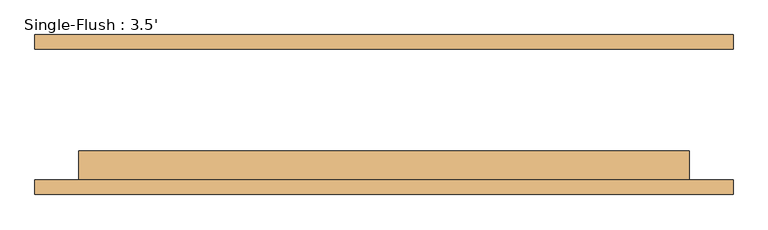
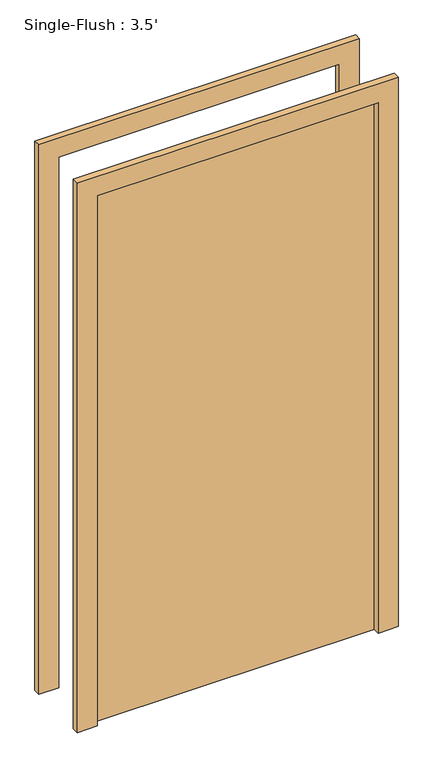
"""IFC4 building model written with IfcOpenShell, lengths in millimetres: door geometry, Single-Flush : 3.5'."""

from ifc_helpers import new_model, si_unit, frame, origin, origin_with_axes, place, context, project, spatial, polyline, outline, extrude, source, transform, mapped, element, save


def single_flush_3_5_0848dd25(model_context):
    return source(origin(), model_context, "Body", "SweptSolid", [
        extrude(outline(polyline([(2209.8, -609.6), (0.0, -609.6), (0.0, -533.4), (2133.6, -533.4), (2133.6, 533.4), (0.0, 533.4), (0.0, 609.6), (2209.8, 609.6), (2209.8, -609.6)])), frame((0.0, -139.7, 0.0), z_axis=(0.0, 1.0, 0.0), x_axis=(0.0, 0.0, 1.0)), (0.0, 0.0, 1.0), 25.4),
        extrude(outline(polyline([(2209.8, 609.6), (2209.8, -609.6), (0.0, -609.6), (0.0, -533.4), (2133.6, -533.4), (2133.6, 533.4), (0.0, 533.4), (0.0, 609.6), (2209.8, 609.6)])), frame((0.0, 114.3, 0.0), z_axis=(0.0, 1.0, 0.0), x_axis=(0.0, 0.0, 1.0)), (0.0, 0.0, 1.0), 25.4),
        extrude(outline(polyline([(533.4, -63.5), (533.4, -114.3), (-533.4, -114.3), (-533.4, -63.5), (533.4, -63.5)])), origin_with_axes(), (0.0, 0.0, 1.0), 2133.6),
    ])


if __name__ == "__main__":
    model = new_model("IFC4")
    model_context = context("Model", 3, world=origin())
    ifc_project = project(units=[si_unit("LENGTHUNIT", "METRE", prefix="MILLI")], contexts=[model_context])
    site = spatial("IfcSite", under=ifc_project)
    building = spatial("IfcBuilding", under=site)
    placement = place(None, origin())
    single_flush_3_5_shape = single_flush_3_5_0848dd25(model_context)
    element("IfcDoor", 1, ObjectType="Single-Flush : 3.5'", at=placement, inside=building, context=model_context, shape_type="MappedRepresentation", body=[
        mapped(single_flush_3_5_shape, transform((0.0, 0.0, 0.0), x_axis=(1.0, 0.0, 0.0), y_axis=(0.0, 1.0, 0.0), z_axis=(0.0, 0.0, 1.0))),
    ])
    save(model, "model.ifc")

# Revit data of these elements
# Type "Single-Flush : 3.5'"
#   Type Mark = "10"
#   Construction Type Id = "MDOOR"
#   Assembly Code = "C1020"
#   Analytic Construction = "Metal"
#   Thickness = 0' - 2"
#   Heat Transfer Coefficient (U) = 0.651978 BTU/(h·ft²·°F)
#   Height = 7' - 0"
#   Trim Projection Ext = 0' - 1"
#   Trim Projection Int = 0' - 1"
#   Trim Width = 0' - 3"
#   Width = 3' - 6"
#   Define Thermal Properties by = 1
#   Door Material = Door - Panel
#   Frame Material = Door - Frame
#   Visual Light Transmittance = 0
#   Solar Heat Gain Coefficient = 0
#   Function = (empty or 0)
#   Wall Closure = (empty or 0)
# Element 1 (IfcDoor, "Single-Flush : 3.5'")
#   Materials on its faces: "Door - Frame", "Door - Panel"
# Materials
#   "Door - Panel": class "Wood", colour RGB 210 159 95, transparency 0
#   "Door - Frame": colour RGB 118 70 51, transparency 0
